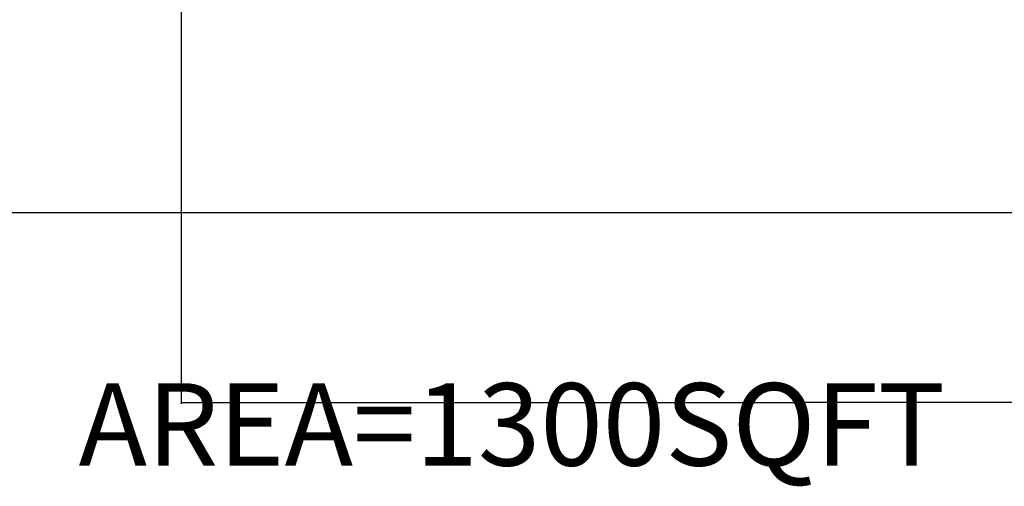
# Model space of a CAD drawing. Units: inches. Extents: x -4347 to -3836, y 955 to 1521.
# Tile 2 of 11: x -4144 to -4001, y 955 to 1023. Entities that reach past the tile are written whole.
import ezdxf

# ---------------------------------------------------------------- set-up
doc = ezdxf.new("R2010")
doc.units = ezdxf.units.IN
doc.header["$MEASUREMENT"] = 0
for name, color, linetype, lineweight in [('A-ANNO-DIMS', 2, 'Continuous', 18), ('A-AREA-IDEN', 7, 'Continuous', 18), ('A-FLOR', 7, 'Continuous', 25)]:
    doc.layers.add(name, color=color, linetype=linetype, lineweight=lineweight)
doc.styles.get("Standard").update_dxf_attribs({"font": 'arial.ttf'})
doc.dimstyles.get("Standard").update_dxf_attribs({"dimtxt": 0.18, "dimasz": 0.18, "dimexe": 0.18, "dimexo": 0.0625, "dimgap": 0.09, "dimtad": 0, "dimtih": 1, "dimtoh": 1, "dimdec": 0, "dimzin": 0, "dimdsep": 46, "dimlunit": 3, "dimtxsty": 'Standard', "dimcen": 0.09, "dimadec": 0, "dimazin": 0, "dimtfac": 1, "dimtdec": 0, "dimtofl": 0, "dimtmove": 0, "dimatfit": 3, "dimfxl": 1, "dimtolj": 1, "dimtzin": 0, "dimarcsym": 0})

# ---------------------------------------------------------------- blocks, each defined once
blk = doc.blocks.new('*D47')
at = {"layer": 'A-ANNO-DIMS', "color": 0, "lineweight": -2, "transparency": 16777216}
for p, q in [((-4120.58, 1288.73), (-4120.58, 966.96)), ((-3940.58, 1288.73), (-3940.58, 966.96)), ((-4120.4, 967.14), (-4030.97, 967.14)), ((-3940.76, 967.14), (-4030.19, 967.14))]:
    blk.add_line(p, q, dxfattribs=at)
at = {"layer": 'A-ANNO-DIMS', "color": 0, "transparency": 16777216}
for points in [[(-4120.4, 967.17), (-4120.4, 967.11), (-4120.58, 967.14)], [(-3940.76, 967.17), (-3940.76, 967.11), (-3940.58, 967.14)]]:
    blk.add_solid(points, dxfattribs=at)
at = {"layer": 'Defpoints', "color": 0, "transparency": 16777216}
for p in [(-4120.58, 1288.79), (-3940.58, 1288.79), (-3940.58, 967.14)]:
    blk.add_point(p, dxfattribs=at)
at = {"layer": 'A-ANNO-DIMS', "color": 0, "transparency": 16777216, "insert": (-4030.58, 967.14), "char_height": 0.18, "attachment_point": 5}
blk.add_mtext('\\A1;15\'-0"', dxfattribs=at)

msp = doc.modelspace()

# ---------------------------------------------------------------- linework, layer by layer
at = {"layer": 'A-FLOR'}
msp.add_line((-4180.58, 994.79), (-3931.58, 994.79), dxfattribs=at)

# ---------------------------------------------------------------- texts
at = {"layer": 'A-AREA-IDEN', "insert": (-4135.5, 969.97), "char_height": 12, "attachment_point": 1}
msp.add_mtext_dynamic_manual_height_columns('AREA=1300SQFT', width=8.7875, gutter_width=1, heights=[0], dxfattribs=at)

# ---------------------------------------------------------------- dimensions: what is measured, and where the dimension line sits
at = {"layer": 'A-ANNO-DIMS'}
dim = msp.add_linear_dim(base=(-3940.58, 967.14), p1=(-4120.58, 1288.79), p2=(-3940.58, 1288.79), dimstyle='Standard', override={"dimdec": 1, "dimlfac": 1, "dimrnd": 0, "dimzin": 1, "dimdsep": 46, "dimlunit": 4, "dimfrac": 2}, dxfattribs=at)
dim.commit()
dim.dimension.update_dxf_attribs({"geometry": '*D47', "text_midpoint": (-4030.58, 967.14)})

doc.saveas('drawing.dxf')
